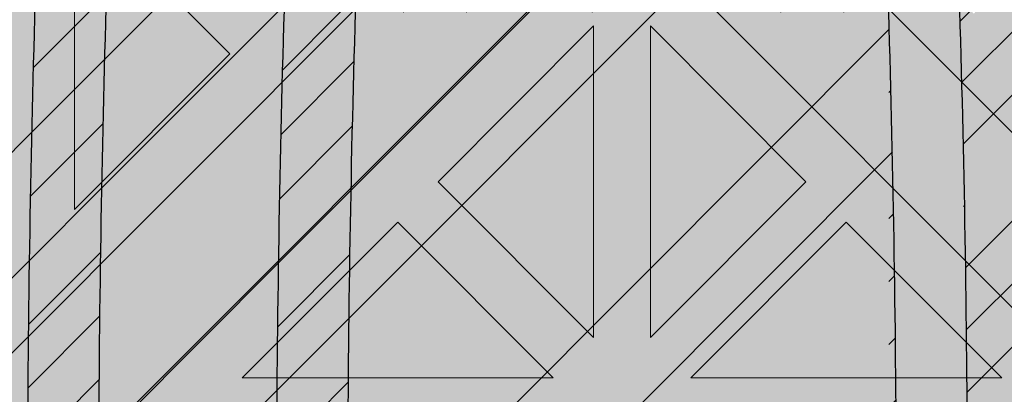
# Model space of a CAD drawing. Units: inches. Extents: x 844 to 2234, y 346 to 1084.
# Tile 60 of 93: x 1866.641 to 1871.054, y 703.938 to 705.614. Entities that reach past the tile are written whole.
import ezdxf

# ---------------------------------------------------------------- set-up
doc = ezdxf.new("R2010")
doc.units = ezdxf.units.IN
doc.header["$MEASUREMENT"] = 0
doc.layers.add('furniture', color=8, linetype='Continuous', lineweight=18)
doc.layers.add('RA-AP-01$0$INT', color=35, linetype='Continuous', lineweight=5)
doc.layers.add('RA-AP-01$0$FURN', color=3, linetype='Continuous')
doc.layers.add('RA-AP-01$0$WOOD', color=64, linetype='Continuous')

# ---------------------------------------------------------------- blocks, each defined once
blk = doc.blocks.new('A$C18D01794')
at = {"layer": 'RA-AP-01$0$INT'}
h = blk.add_hatch(color=256, dxfattribs=at)
h.paths.add_polyline_path([(4.585917135068448, -7.856712009587804), (4.614201406330596, -7.856712009587056), (4.668846067270487, -7.802067348644738), (4.723490728212344, -7.856712009584164), (4.771774999457151, -7.856712009582887), (4.826419660396886, -7.80206734864072), (4.862780050090322, -7.838427738332541), (4.844495778842715, -7.856712009580965), (4.862780050090411, -7.856712009580482), (4.905206456960182, -7.814285602707865), (4.947632863832445, -7.856712009578238), (4.965917135079675, -7.856712009577755), (4.947632863831759, -7.838427738330656), (4.983993253523576, -7.802067348637219), (5.038637914464627, -7.856712009575829), (5.08692218571208, -7.856712009574554), (5.141566846649976, -7.802067348634224), (5.196211507589851, -7.856712009571666), (5.224495778822615, -7.856712009570916), (4.905206456953975, -7.537422687702283)])
h.paths.add_polyline_path([(4.895206456956031, -7.575706958950402), (4.895206456958921, -7.684996280828174), (4.840561796018589, -7.630351619890275)], flags=16)
h.paths.add_polyline_path([(4.915206456955638, -7.575706958949956), (4.969851117895509, -7.630351619887399), (4.915206456957609, -7.684996280827732)], flags=16)
h.paths.add_polyline_path([(4.826419660395175, -7.644493755514321), (4.881064321335613, -7.699138416452331), (4.771774999456703, -7.69913841645522)], flags=16)
h.paths.add_polyline_path([(4.983993253519558, -7.644493755510815), (5.038637914460456, -7.699138416449285), (4.929348592581548, -7.69913841645126)], flags=16)
h.paths.add_polyline_path([(4.881064321336025, -7.719138416452334), (4.826419660397532, -7.773783077393256), (4.771774999457062, -7.719138416455217)], flags=16)
h.paths.add_polyline_path([(4.929348592582019, -7.71913841645126), (5.038637914460982, -7.719138416449284), (4.983993253522945, -7.773783077389749)], flags=16)
h.paths.add_polyline_path([(4.895206456960191, -7.733280552075633), (4.895206456962115, -7.806001331460164), (4.876922185715016, -7.824285602708492), (4.840561796021581, -7.787925213016675)], flags=16)
h.paths.add_polyline_path([(4.915206456958487, -7.733280552075187), (4.969851117899527, -7.787925213013798), (4.933490728206909, -7.824285602708034), (4.9152064569598, -7.806001331461736)], flags=16)
h.paths.add_polyline_path([(4.757632863832376, -7.733280552079264), (4.812277524772842, -7.787925213017304), (4.757632863834348, -7.842569873958233)], flags=16)
h.paths.add_polyline_path([(4.737632863832376, -7.73328055207979), (4.737632863834348, -7.842569873958701), (4.682988202893906, -7.787925213020692)], flags=16)
h.paths.add_polyline_path([(5.05278005008503, -7.733280552072701), (5.052780050087917, -7.842569873951664), (4.998135389146995, -7.787925213013169)], flags=16)
h.paths.add_polyline_path([(5.072780050085024, -7.733280552072333), (5.127424711025931, -7.787925213010806), (5.072780050087916, -7.842569873951244)], flags=16)
h.paths.add_polyline_path([(4.935917135072783, -7.506712009583784), (5.255206456948811, -7.826001331459767), (5.255206456948932, -7.797717060211899), (5.200561796010279, -7.743072399273238), (5.255206456949403, -7.688427738334128), (5.25520645694961, -7.640143467086677), (5.200561796009787, -7.585498806146837), (5.236922185702417, -7.549138416454212), (5.255206456949919, -7.56742268770172), (5.255206456949998, -7.549138416454178), (5.212780050078687, -7.506712009583814), (5.25520645695036, -7.464285602712145), (5.255206456950438, -7.446001331464763), (5.236922185702424, -7.464285602712779), (5.200561796009796, -7.427925213020149), (5.255206456950753, -7.373280552079203), (5.25520645695096, -7.324996280834394), (5.200561796010322, -7.270351619893748), (5.255206456951428, -7.215706958952649), (5.255206456951547, -7.187422687705071)])
h.paths.add_polyline_path([(5.042988202883395, -7.42792521302065), (5.097632863823085, -7.373280552080975), (5.097632863822622, -7.482569873959883)], flags=16)
h.paths.add_polyline_path([(5.028846067259663, -7.442067348644384), (5.083490728198774, -7.496712009583504), (4.974201406321001, -7.496712009583035)], flags=16)
h.paths.add_polyline_path([(5.117632863823087, -7.37328055208089), (5.172277524762331, -7.42792521302015), (5.11763286382262, -7.482569873959851)], flags=16)
h.paths.add_polyline_path([(5.08349072819877, -7.516712009582191), (5.028846067259652, -7.571356670521302), (4.974201406320998, -7.516712009582638)], flags=16)
h.paths.add_polyline_path([(5.131774999446817, -7.35913841645716), (5.186419660386065, -7.413783077396415), (5.241064321325782, -7.359138416456712)], flags=17)
h.paths.add_polyline_path([(5.131774999446228, -7.496712009583703), (5.186419660386065, -7.442067348643883), (5.222780050079488, -7.478427738337313), (5.204495778832781, -7.496712009584014)], flags=16)
h.paths.add_polyline_path([(5.097632863822613, -7.530854145205813), (5.097632863823061, -7.640143467084723), (5.042988202883383, -7.585498806145032)], flags=16)
h.paths.add_polyline_path([(5.131774999446899, -7.339138416457162), (5.241064321325809, -7.339138416456712), (5.186419660386591, -7.284493755517479)], flags=17)
h.paths.add_polyline_path([(5.131774999446226, -7.516712009581999), (5.204495778830767, -7.516712009581702), (5.22278005007868, -7.534996280829206), (5.186419660386049, -7.571356670521828)], flags=16)
h.paths.add_polyline_path([(5.11763286382262, -7.530854145205852), (5.17227752476232, -7.585498806145562), (5.117632863823064, -7.64014346708481)], flags=16)
h.paths.add_polyline_path([(5.186419660386069, -7.599640941770585), (5.241064321325754, -7.654285602710281), (5.131774999446791, -7.654285602709814)], flags=16)
h.paths.add_polyline_path([(5.131774999446872, -7.674285602709813), (5.24106432132578, -7.674285602710282), (5.186419660386554, -7.728930263649504)], flags=16)
h.paths.add_polyline_path([(5.255206456951811, -7.126001331467467), (5.255206456951895, -7.106712009588038), (4.555206456956052, -7.106712009588038), (4.555206456956136, -7.12600133146746), (4.905206456953973, -7.476001331465289)])
h.paths.add_polyline_path([(4.983993253513404, -7.368930263651977), (4.92934859257295, -7.314285602713969), (5.03863791445186, -7.314285602711063)], flags=16)
h.paths.add_polyline_path([(4.969851117889988, -7.383072399276016), (4.915206456952556, -7.437717060215906), (4.915206456949648, -7.328427738338133)], flags=16)
h.paths.add_polyline_path([(4.929348592572535, -7.294285602713971), (4.983993253511019, -7.239640941773039), (5.038637914451496, -7.294285602711065)], flags=16)
h.paths.add_polyline_path([(5.052780050074912, -7.280143467087016), (4.998135389134438, -7.225498806148989), (5.052780050072919, -7.170854145208052)], flags=16)
h.paths.add_polyline_path([(5.07278005007491, -7.280143467086489), (5.072780050072918, -7.170854145207579), (5.127424711013374, -7.225498806145578)], flags=16)
h.paths.add_polyline_path([(4.89520645695295, -7.437717060216355), (4.840561796013067, -7.383072399278919), (4.895206456950961, -7.328427738338582)], flags=16)
h.paths.add_polyline_path([(4.915206456948365, -7.280143467090674), (4.915206456946434, -7.207422687704125), (4.933490728192729, -7.18913841645701), (4.969851117886972, -7.225498806149623)], flags=16)
h.paths.add_polyline_path([(4.881064321327021, -7.314285602715054), (4.82641966038902, -7.368930263655506), (4.771774999448108, -7.314285602717047)], flags=16)
h.paths.add_polyline_path([(4.895206456950073, -7.280143467091125), (4.840561796009022, -7.225498806152518), (4.876922185700835, -7.18913841645908), (4.895206456948749, -7.207422687706589)], flags=16)
h.paths.add_polyline_path([(4.983993253510392, -7.211356670525576), (4.947632863816944, -7.174996280833758), (4.965917135064043, -7.156712009585847), (5.038637914448995, -7.156712009584522)], flags=16)
h.paths.add_polyline_path([(4.881064321326543, -7.294285602715056), (4.771774999447578, -7.294285602717046), (4.826419660385607, -7.239640941776569)], flags=16)
h.paths.add_polyline_path([(4.905206456946447, -7.19913841645844), (4.862780050074785, -7.156712009587725), (4.947632863816685, -7.156712009586302)], flags=16)
h.paths.add_polyline_path([(5.14156684663679, -7.211356670521528), (5.086922185696452, -7.156712009583639), (5.196211507574223, -7.156712009581651)], flags=16)
h.paths.add_polyline_path([(4.8264196603837, -7.211356670529104), (4.771774999442643, -7.156712009590501), (4.8444957788276, -7.156712009588568), (4.862780050075511, -7.17499628083566)], flags=16)
h.paths.add_polyline_path([(4.812277524760289, -7.225498806153156), (4.757632863822258, -7.28014346709363), (4.757632863819352, -7.170854145214669)], flags=16)
h.paths.add_polyline_path([(4.73763286382226, -7.280143467093997), (4.682988202881349, -7.22549880615554), (4.737632863819352, -7.170854145215086)], flags=16)
h.paths.add_polyline_path([(4.723490728195188, -7.156712009591787), (4.668846067257299, -7.211356670532127), (4.614201406317417, -7.156712009594693)], flags=16)
h.paths.add_polyline_path([(4.597632863829262, -7.506712009583814), (4.555206456957951, -7.54913841645418), (4.555206456958029, -7.56742268770172), (4.573490728205535, -7.549138416454212), (4.609851117898167, -7.585498806146839), (4.555206456958338, -7.640143467086675), (4.555206456958546, -7.688427738334125), (4.60985111789767, -7.743072399273238), (4.555206456959015, -7.797717060211899), (4.555206456959138, -7.826001331459767), (4.874495778835167, -7.506712009583786), (4.5552064569564, -7.187422687705062), (4.555206456956523, -7.215706958952644), (4.609851117897629, -7.270351619893746), (4.555206456956988, -7.324996280834396), (4.555206456957198, -7.373280552079195), (4.609851117898153, -7.427925213020147), (4.573490728205528, -7.464285602712779), (4.555206456957507, -7.446001331464756), (4.555206456957585, -7.464285602712143)])
h.paths.add_polyline_path([(4.712780050085332, -7.482569873959882), (4.712780050084863, -7.373280552080972), (4.767424711024555, -7.42792521302065)], flags=16)
h.paths.add_polyline_path([(4.726922185709173, -7.496712009583504), (4.781566846648288, -7.442067348644384), (4.836211507586949, -7.496712009583033)], flags=16)
h.paths.add_polyline_path([(4.692780050085327, -7.482569873959851), (4.638135389145619, -7.427925213020149), (4.692780050084865, -7.373280552080892)], flags=16)
h.paths.add_polyline_path([(4.726922185709182, -7.516712009582191), (4.836211507586949, -7.51671200958264), (4.7815668466483, -7.571356670521304)], flags=16)
h.paths.add_polyline_path([(4.678637914461726, -7.496712009583706), (4.605917135075169, -7.496712009584014), (4.587632863828464, -7.478427738337311), (4.623993253521887, -7.442067348643881)], flags=16)
h.paths.add_polyline_path([(4.712780050085336, -7.530854145205816), (4.767424711024568, -7.585498806145034), (4.71278005008489, -7.640143467084724)], flags=16)
h.paths.add_polyline_path([(4.678637914461726, -7.516712009582001), (4.623993253521899, -7.571356670521829), (4.587632863829271, -7.534996280829206), (4.605917135077185, -7.5167120095817)], flags=16)
h.paths.add_polyline_path([(4.692780050085336, -7.530854145205848), (4.692780050084889, -7.64014346708481), (4.638135389145632, -7.585498806145562)], flags=16)
h.paths.add_polyline_path([(4.623993253521885, -7.413783077396415), (4.678637914461131, -7.359138416457161), (4.56934859258217, -7.359138416456712)], flags=17)
h.paths.add_polyline_path([(4.623993253521901, -7.599640941770568), (4.678637914461158, -7.654285602709814), (4.569348592582195, -7.654285602710281)], flags=16)
h.paths.add_polyline_path([(4.678637914461051, -7.339138416457162), (4.623993253521361, -7.284493755517479), (4.569348592582143, -7.339138416456712)], flags=17)
h.paths.add_polyline_path([(4.678637914461076, -7.674285602709813), (4.623993253521399, -7.728930263649504), (4.569348592582167, -7.674285602710281)], flags=16)
h = blk.add_hatch(color=256, dxfattribs=at)
h.paths.add_polyline_path([(4.905206456954232, -7.537422687702028), (4.874495778835232, -7.506712009583718), (4.555206456959138, -7.826001331459766), (4.555206456959269, -7.856712009588616), (4.585917135068449, -7.856712009587804)])
h.paths.add_polyline_path([(4.935917135072152, -7.506712009583152), (4.905206456953497, -7.537422687701806), (5.224495778822614, -7.856712009570917), (5.255206456948681, -7.856712009570104), (5.255206456948813, -7.826001331459768)])
h.paths.add_polyline_path([(5.255206456951549, -7.18742268770507), (5.255206456951813, -7.126001331467461), (4.905206456953563, -7.476001331465701), (4.935917135072559, -7.506712009584006)])
h.paths.add_polyline_path([(4.874495778835167, -7.506712009583785), (4.905206456953818, -7.476001331465132), (4.555206456956135, -7.126001331467458), (4.555206456956399, -7.187422687705064)])
h = blk.add_hatch(color=256, dxfattribs=at)
h.paths.add_polyline_path([(4.89520645695096, -7.328427738338579), (4.840561796013068, -7.383072399278921), (4.89520645695295, -7.437717060216353)])
h.paths.add_polyline_path([(4.915206456952557, -7.437717060215907), (4.969851117889986, -7.383072399276024), (4.915206456949648, -7.328427738338133)])
h.paths.add_polyline_path([(4.929348592572952, -7.31428560271397), (4.983993253513403, -7.368930263651974), (5.038637914451863, -7.314285602711064)])
h.paths.add_polyline_path([(5.038637914451498, -7.294285602711065), (4.983993253511018, -7.239640941773039), (4.929348592572535, -7.294285602713969)])
h.paths.add_polyline_path([(4.969851117886971, -7.225498806149624), (4.93349072819273, -7.189138416457011), (4.915206456946433, -7.207422687704124), (4.915206456948367, -7.280143467090678)])
h.paths.add_polyline_path([(4.965917135064045, -7.156712009585847), (4.947632863816945, -7.17499628083376), (4.983993253510389, -7.211356670525573), (5.038637914448995, -7.156712009584522)])
h.paths.add_polyline_path([(4.998135389134439, -7.22549880614899), (5.05278005007491, -7.280143467087016), (5.052780050072921, -7.170854145208054)])
h.paths.add_polyline_path([(5.072780050074911, -7.28014346708649), (5.127424711013374, -7.225498806145579), (5.072780050072921, -7.170854145207581)])
h.paths.add_polyline_path([(5.196211507574225, -7.156712009581651), (5.08692218569645, -7.156712009583639), (5.141566846636789, -7.211356670521529)])
h.paths.add_polyline_path([(4.862780050074782, -7.156712009587723), (4.90520645694645, -7.199138416458444), (4.94763286381669, -7.156712009586302)])
h.paths.add_polyline_path([(4.895206456950073, -7.280143467091126), (4.895206456948746, -7.207422687706587), (4.876922185700836, -7.189138416459078), (4.840561796009025, -7.225498806152521)])
h.paths.add_polyline_path([(4.826419660385605, -7.239640941776569), (4.771774999447577, -7.294285602717049), (4.881064321326541, -7.294285602715055)])
h.paths.add_polyline_path([(4.771774999448108, -7.314285602717046), (4.82641966038902, -7.368930263655505), (4.88106432132702, -7.314285602715054)])
h.paths.add_polyline_path([(4.757632863822258, -7.280143467093631), (4.812277524760285, -7.225498806153153), (4.757632863819352, -7.170854145214668)])
h.paths.add_polyline_path([(4.862780050075512, -7.17499628083566), (4.844495778827599, -7.156712009588567), (4.771774999442647, -7.156712009590504), (4.8264196603837, -7.211356670529104)])
h.paths.add_polyline_path([(4.682988202881349, -7.225498806155537), (4.737632863822258, -7.280143467093997), (4.737632863819352, -7.170854145215087)])
h.paths.add_polyline_path([(4.723490728195189, -7.156712009591783), (4.614201406317418, -7.156712009594692), (4.668846067257298, -7.211356670532127)])
h = blk.add_hatch(color=256, dxfattribs=at)
h.paths.add_polyline_path([(4.781566846647504, -7.442067348645805), (4.836211507586161, -7.496712009584463), (4.726922185708388, -7.496712009584918)])
h.paths.add_polyline_path([(4.836211507586161, -7.516712009584068), (4.781566846647504, -7.571356670522723), (4.726922185708388, -7.516712009583606)])
h.paths.add_polyline_path([(4.76742471102377, -7.585498806146453), (4.712780050084083, -7.640143467086137), (4.712780050084542, -7.530854145207227)])
h.paths.add_polyline_path([(4.692780050084544, -7.530854145207257), (4.692780050084084, -7.64014346708622), (4.638135389144834, -7.585498806146965)])
h.paths.add_polyline_path([(4.678637914460932, -7.516712009583407), (4.623993253521102, -7.571356670523233), (4.587632863827676, -7.53499628082981), (4.605917135074382, -7.516712009583104)])
h.paths.add_polyline_path([(4.573490728204743, -7.54913841645434), (4.60985111789737, -7.585498806146969), (4.555206456957541, -7.640143467086797), (4.555206456957237, -7.567422687701846)])
h.paths.add_polyline_path([(4.623993253521098, -7.599640941770699), (4.67863791446035, -7.654285602709951), (4.56934859258139, -7.654285602710407)])
h.paths.add_polyline_path([(4.678637914460275, -7.67428560270995), (4.623993253520583, -7.728930263649637), (4.56934859258136, -7.674285602710405)])
h.paths.add_polyline_path([(4.609851117896854, -7.743072399273369), (4.555206456958196, -7.797717060212026), (4.555206456957738, -7.688427738334254)])
h.paths.add_polyline_path([(4.597632863828475, -7.506712009583301), (4.555206456957283, -7.549138416454495), (4.555206456956805, -7.464285602712587)])
h.paths.add_polyline_path([(4.678637914460932, -7.496712009585113), (4.605917135076396, -7.496712009585417), (4.587632863828479, -7.478427738337913), (4.623993253521104, -7.442067348645284)])
h.paths.add_polyline_path([(4.692780050084091, -7.373280552082301), (4.692780050084548, -7.482569873961267), (4.638135389144834, -7.427925213021552)])
h.paths.add_polyline_path([(4.767424711023772, -7.427925213022072), (4.712780050084545, -7.48256987396129), (4.712780050084089, -7.373280552082384)])
h.paths.add_polyline_path([(4.67863791446036, -7.359138416457298), (4.623993253521105, -7.41378307739655), (4.569348592581399, -7.35913841645684)])
h.paths.add_polyline_path([(4.609851117897371, -7.427925213020278), (4.573490728204743, -7.464285602712907), (4.555206456957237, -7.446001331465401), (4.555206456957548, -7.373280552080448)])
h.paths.add_polyline_path([(4.623993253520596, -7.284493755517612), (4.67863791446028, -7.339138416457299), (4.569348592581367, -7.339138416456838)])
h.paths.add_polyline_path([(4.609851117896867, -7.270351619893878), (4.555206456957749, -7.324996280832994), (4.55520645695821, -7.21570695895522)])
for p, q in [((4.905206456953975, -7.476001331465289), (4.555206456956136, -7.12600133146746)), ((4.905206456953975, -7.476001331465289), (5.255206456951811, -7.126001331467465)), ((4.874495778835167, -7.506712009583786), (4.555206456956399, -7.187422687705064)), ((4.935917135072783, -7.506712009583784), (5.255206456951548, -7.187422687705069)), ((4.771774999448109, -7.314285602717045), (4.881064321327019, -7.314285602715054)), ((4.826419660389018, -7.368930263655503), (4.771774999448109, -7.314285602717045)), ((4.881064321327019, -7.314285602715054), (4.82641966038902, -7.368930263655505)), ((4.929348592572952, -7.314285602713971), (4.983993253513403, -7.368930263651975)), ((5.038637914451862, -7.314285602711064), (4.929348592572952, -7.314285602713971)), ((4.983993253513404, -7.368930263651973), (5.038637914451862, -7.314285602711064)), ((4.895206456950956, -7.328427738338584), (4.840561796013068, -7.383072399278921)), ((4.895206456950959, -7.328427738338582), (4.89520645695295, -7.437717060216353)), ((4.915206456949651, -7.328427738338136), (4.969851117889986, -7.383072399276024)), ((4.915206456949648, -7.328427738338135), (4.915206456952556, -7.437717060215906)), ((4.767424711024554, -7.42792521302065), (4.712780050084865, -7.373280552080972)), ((4.712780050084865, -7.373280552080972), (4.71278005008533, -7.482569873959882)), ((4.89520645695295, -7.437717060216353), (4.840561796013068, -7.383072399278921)), ((4.915206456952556, -7.437717060215906), (4.969851117889986, -7.383072399276024)), ((4.71278005008533, -7.482569873959882), (4.767424711024555, -7.427925213020651))]:
    blk.add_line(p, q, dxfattribs=at)
blk = doc.blocks.new('A$C32926AE1')
at = {"layer": 'RA-AP-01$0$FURN'}
h = blk.add_hatch(dxfattribs=at)
h.set_pattern_fill('ANSI31', color=256, scale=0.1, style=0)
h.set_pattern_definition([(45, (0, 0), (-0.0088388347648318, 0.0088388347648318), [])])
edge = h.paths.add_edge_path(flags=16)
edge.add_arc((4.904771284329206, 4.246793130718756), 0.2603971832811541, 75.22398030683196, 104.7760196931204)
edge.add_arc((4.904771284329206, 4.246793130718756), 0.2603971832811541, 75.223980306832, 104.77601969312039, ccw=False)
edge = h.paths.add_edge_path(flags=16)
edge.add_arc((4.904771284329206, 4.067062675376612), 0.2603971832811541, 255.2239803068796, 284.776019693168)
edge.add_arc((4.904771284329206, 4.067062675376612), 0.2603971832811541, 255.22398030687958, 284.77601969316805, ccw=False)
edge = h.paths.add_edge_path(flags=0)
edge.add_arc((4.904771284329206, 4.067062675376612), 0.2603971832811541, 255.2239803068796, 284.776019693168)
edge.add_arc((4.904771284329206, 4.067062675376612), 0.2603971832811541, 255.22398030687958, 284.77601969316805, ccw=False)
edge = h.paths.add_edge_path(flags=0)
edge.add_arc((4.904771284329206, 4.067062675376612), 0.2603971832811541, 255.2239803068796, 284.776019693168)
edge.add_arc((4.904771284329206, 4.067062675376612), 0.2603971832811541, 255.22398030687958, 284.77601969316805, ccw=False)
edge = h.paths.add_edge_path()
edge.add_arc((4.604388392048174, 4.588829985554312), 0.1599999999999918, 342.3781640246255, 354.4317409793762)
edge.add_arc((5.090145208887507, 4.43216705527679), 0.3503971832811637, 162.0091218307731, 180.3186872093483)
edge.add_arc((5.205154176610243, 4.588829985554953), 0.1599999999999917, 185.5682590208461, 197.6218359767349)
edge.add_arc((4.904771284329229, 4.246793130718735), 0.3503971832811761, 72.00912183053516, 107.9908781690354)
edge.add_arc((9.535952835716557, 4.28682295566602), 4.798342501046485, 178.2875002453811, 181.5576802719453)
edge.add_arc((4.719397359771122, 4.43216705527679), 0.3503971832811637, 359.6813127906516, 377.9908781692269)
edge.add_arc((9.535967292294904, 4.286822350292874), 4.778371420254705, 178.2965938931842, 181.5667745797229)
edge.add_arc((4.719397359771122, 4.43216705527679), 0.3303971832811637, 359.6813127906516, 377.9908781692269)
edge.add_arc((0.2735752763637294, 4.286822350292874), 4.7783714202547, 358.4332254202771, 361.7034061068158)
edge.add_arc((5.061434214606998, 4.732549947558029), 0.1600000000000254, 252.3781640250584, 264.4317409792362)
edge.add_arc((4.748108354051257, 4.732549947558012), 0.1600000000000541, 275.5682590208426, 287.6218359759532)
edge.add_arc((4.604388392048115, 4.588829985554317), 0.1800000000000505, 342.3567572500182, 349.3735009646207)
edge.add_arc((5.205154176610254, 4.588829985554976), 0.1800000000000069, 190.6264990356027, 197.6432427513933)
edge.add_arc((5.061434214607106, 4.732549947558013), 0.1800000000000424, 252.3567572496606, 259.3735009644582)
edge.add_arc((4.904771284329208, 4.246793130718737), 0.3303971832811676, 71.99844483668534, 108.0015551637021)
edge.add_arc((4.748108354051414, 4.732549947558045), 0.1800000000000547, 280.6264990355479, 287.6432427495938)
edge.add_arc((5.090145208887514, 4.432167055276789), 0.2803971832811691, 162.8706300666893, 180.816523289902)
edge.add_arc((4.719397359771136, 4.432167055276689), 0.2803971832811534, 359.183476710103, 377.1293699333214)
edge.add_arc((4.904771284329222, 4.246793130718737), 0.2803971832811769, 72.87063006672916, 107.1293699332334)
edge.add_arc((5.090145208887522, 4.432167055276788), 0.2603971832811776, 165.2239803068007, 180.9953123810312)
edge.add_arc((4.719397359771141, 4.432167055276699), 0.2603971832811458, 359.0046876189768, 374.7760196932087)
edge.add_arc((5.090145208887507, 4.43216705527679), 0.3303971832811637, 162.0091218307731, 180.3186872093483)
edge.add_arc((9.53595427642584, 4.285015535491528), 4.728345371032053, 178.265043920078, 181.5679956281801)
edge.add_arc((0.2735882922327999, 4.285015535491582), 4.728345371032045, 358.4320043718193, 361.7349560799204)
edge.add_arc((9.535953591267507, 4.284458026472751), 4.708343996644348, 178.2573054306777, 181.5704995759608)
edge.add_arc((0.273588977391114, 4.284458026472785), 4.708343996644358, 358.4295004240388, 361.7426945693213)
edge.add_arc((0.2735889773911131, 4.029397779622582), 4.708343996644359, 358.2573054306787, 361.5704995759613)
edge.add_arc((9.535953591267518, 4.029397779622618), 4.708343996644359, 178.4295004240391, 181.7426945693223)
edge.add_arc((0.2735882922327901, 4.028840270603786), 4.728345371032054, 358.2650439200796, 361.5679956281808)
edge.add_arc((9.53595427642584, 4.028840270603841), 4.728345371032054, 178.4320043718199, 181.7349560799219)
edge.add_arc((0.2735752763637302, 4.027033455802493), 4.778371420254699, 358.2965938931842, 361.5667745797229)
edge.add_arc((4.719397359771122, 3.881688750818578), 0.3303971832811637, 342.0091218307731, 360.3186872093484)
edge.add_arc((5.090145208887507, 3.881688750818578), 0.3303971832811637, 179.6813127906516, 197.9908781692269)
edge.add_arc((9.535967292294904, 4.027033455802493), 4.778371420254705, 178.433225420277, 181.7034061068158)
edge.add_arc((4.719397359771122, 3.881688750818578), 0.3503971832811637, 342.0091218307731, 360.3186872093484)
edge.add_arc((9.53595283571655, 4.027032850429349), 4.79834250104648, 178.4423197280546, 181.7124997546188)
edge.add_arc((4.719397359771141, 3.881688750818669), 0.2603971832811458, 345.2239803067913, 360.9953123810232)
edge.add_arc((5.090145208887522, 3.88168875081858), 0.2603971832811776, 179.0046876189687, 194.7760196931993)
edge.add_arc((4.904771284329222, 4.067062675376631), 0.2803971832811769, 252.8706300667665, 287.1293699332708)
edge.add_arc((4.719397359771136, 3.881688750818678), 0.2803971832811534, 342.8706300666787, 360.8165232898969)
edge.add_arc((5.090145208887514, 3.881688750818579), 0.2803971832811691, 179.183476710098, 197.1293699333106)
edge.add_arc((4.748108354051414, 3.581305858537323), 0.1800000000000547, 72.3567572504062, 79.37350096445199)
edge.add_arc((4.904771284329208, 4.067062675376631), 0.3303971832811676, 251.9984448362979, 288.0015551633146)
edge.add_arc((5.061434214607106, 3.581305858537355), 0.1800000000000424, 100.6264990355418, 107.6432427503394)
edge.add_arc((5.205154176610254, 3.725025820540392), 0.1800000000000069, 162.3567572486066, 169.3735009643972)
edge.add_arc((4.604388392048115, 3.725025820541051), 0.1800000000000505, 10.62649903537925, 17.64324274998182)
edge.add_arc((4.748108354051257, 3.581305858537356), 0.1600000000000541, 72.37816402404681, 84.43174097915735)
edge.add_arc((4.904771284329229, 4.067062675376632), 0.3503971832811761, 252.0091218309645, 287.9908781694648)
edge.add_arc((5.061434214606998, 3.581305858537339), 0.1600000000000254, 95.56825902076373, 107.6218359749416)
edge.add_arc((5.205154176610243, 3.725025820540414), 0.1599999999999917, 162.3781640232651, 174.4317409791539)
edge.add_arc((5.090145208887507, 3.881688750818578), 0.3503971832811637, 179.6813127906516, 197.9908781692269)
edge.add_arc((4.604388392048174, 3.725025820541056), 0.1599999999999918, 5.568259020623824, 17.62183597537444)
edge.add_arc((0.2735897329420762, 4.28682295566602), 4.798342501046482, 358.4423197280547, 361.7124997546188)
edge.add_arc((0.2735897329420691, 4.027032850429348), 4.798342501046489, 358.2875002453812, 361.5576802719453)
at = {"layer": 'RA-AP-01$0$WOOD'}
h = blk.add_hatch(color=256, dxfattribs=at)
h.dxf.hatch_style = 1
h.paths.add_polyline_path([(5.157430609644524, 4.573483066760929, -0.1009492694046607), (5.155401577623758, 4.593365984175333, -0.1842662638101597), (5.172249623284174, 4.638795604568598, 0.2056608120311276), (5.179560981299304, 4.661316324430096, 0.3614336704623542), (5.134352340494423, 4.706524965234944, 0.2056608120311297), (5.111831620632933, 4.699213607219793, -0.1842662638101113), (5.066402000239693, 4.682365561559342, -0.1055311479399994), (5.045656153913092, 4.68467289944697, 0.1567636581983829), (4.763886414745334, 4.684672899446966, -0.1055311479399895), (4.743140568418733, 4.68236556155934, -0.1842662638100833), (4.6977109480255, 4.69921360721979, 0.2056608120302612), (4.675190228164109, 4.706524965234949, 0.3614336704708441), (4.629981587358889, 4.66131632442871, 0.2056608120245944), (4.637292945374126, 4.638795604567974, -0.1842662638101024), (4.654140991034615, 4.59336598417475, -0.1009492694055169), (4.652111959013835, 4.573483066760181, 0.021410119221476), (4.629748025606143, 4.156712009541676, 0.0214101192214795), (4.652111959013809, 3.739940952323101, -0.1009492694059586), (4.654140991034615, 3.720058034908448, -0.1842662638100975), (4.637292945374126, 3.674628414515226, 0.2056608120245705), (4.629981587358889, 3.652107694654492, 0.3614336704708879), (4.675190228164113, 3.606899053848249, 0.2056608120302384), (4.697710948025501, 3.614210411863408, -0.1842662638100995), (4.743140568418738, 3.63105845752386, -0.1055311479402541), (4.763886414745388, 3.628751119636215, 0.1567636581983776), (5.045656153913137, 3.628751119636244, -0.1055311479397538), (5.066402000239692, 3.631058457523857, -0.1842662638101067), (5.111831620632931, 3.614210411863407, 0.2056608120310924), (5.134352340494417, 3.606899053848256, 0.3614336704624001), (5.179560981299307, 3.652107694653103, 0.2056608120311314), (5.172249623284175, 3.6746284145146, -0.1842662638101402), (5.155401577623758, 3.72005803490786, -0.1009492694051366), (5.15743060964455, 3.739940952322354, 0.0214101192215073), (5.179794543052287, 4.156712009541468, 0.0214101192215252)])
h.paths.add_polyline_path([(4.639748609479751, 4.156712009541513, 0.0213537860821624), (4.661970494867118, 3.741887061152232, -0.094075836301374), (4.664143710413708, 3.7196126951003, -0.1824818158568985), (4.644813765429836, 3.668037719127816, 0.2056608120245319), (4.639939526753007, 3.653023905887301, 0.3614336704710246), (4.676106439397173, 3.616856993242342, 0.2056608120302234), (4.691120252638095, 3.621731231919122, -0.1824818158602558), (4.742695228611606, 3.641061176902986, -0.1029891339458722), (4.766991894714349, 3.638256818950944, 0.156709409989566), (5.042550673941472, 3.638256818950105, -0.102989133958497), (5.066847340047078, 3.641061176902949, -0.1824818158594995), (5.118422316020358, 3.621731231919103, 0.2056608120311416), (5.133436129261316, 3.616856993242346, 0.3614336704621468), (5.169603041905217, 3.653023905886178, 0.2056608120310986), (5.164728803228477, 3.668037719127177, -0.1824818158565612), (5.145398858244737, 3.719612695099578, -0.0940758363009313), (5.147572073791232, 3.741887061151398, 0.0213537860822023), (5.169793959178681, 4.156712009541451, 0.0213537860822226), (5.147572073791203, 4.571536957931898, -0.0940758363005034), (5.145398858244737, 4.59381132398362, -0.1824818158565587), (5.164728803228476, 4.645386299956021, 0.2056608120311045), (5.169603041905216, 4.66040011319702, 0.3614336704621845), (5.133436129261313, 4.696567025840856, 0.2056608120310773), (5.118422316020359, 4.691692787164098, -0.182481815859508), (5.066847340047078, 4.67236284218025, -0.1029891339584606), (5.04255067394148, 4.675167200133092, 0.156709409989566), (4.766991894714357, 4.675167200132257, -0.1029891339458842), (4.742695228611611, 4.672362842180213, -0.1824818158602725), (4.691120252638095, 4.691692787164077, 0.2056608120302152), (4.676106439397174, 4.696567025840858, 0.3614336704710363), (4.639939526753005, 4.660400113195899, 0.2056608120245495), (4.644813765429837, 4.645386299955384, -0.1824818158568934), (4.664143710413708, 4.593811323982902, -0.0940758363009187), (4.661970494867149, 4.571536957931074, 0.021353786082177)], flags=16)
h.paths.add_polyline_path([(5.129794543052235, 4.432167055276933, -0.0141661062790638), (5.130152669293814, 4.156927903047693, -0.0141661062790647), (5.129794543052234, 3.881688750818433, -0.0785247771143638), (5.10979738006795, 3.755143611847103, 0.0945969212073497), (5.105408519571111, 3.717898134952927, 0.1043170707844957), (5.116074640131521, 3.670385395016088, 0.1043170707864965), (5.068561900193738, 3.681051515576561, 0.09459692119553), (5.031316423304057, 3.676662655080835, -0.1580239521427272), (4.778226145355827, 3.676662655080367, 0.0945969211986668), (4.740980668464973, 3.681051515576592, 0.1043170707882822), (4.693467928526415, 3.670385395015844, 0.1043170707867916), (4.704134049087309, 3.717898134953662, 0.0945969211972894), (4.69974518859162, 3.755143611844042, -0.0785247771163196), (4.679748025606343, 3.881688750818406, -0.0141661062790663), (4.679389899364763, 4.156927903047693, -0.0141661062790672), (4.679748025606343, 4.432167055276998, -0.0785247771163064), (4.699745188591625, 4.55871219425134, 0.094596921197333), (4.704134049087308, 4.595957671141738, 0.1043170707867205), (4.693467928526416, 4.643470411079523, 0.1043170707882628), (4.740980668464965, 4.632804290518776, 0.0945969211988114), (4.778226145355874, 4.637193151015016, -0.158023952142669), (5.031316423304015, 4.637193151014546, 0.0945969211956361), (5.068561900193736, 4.632804290518806, 0.1043170707864979), (5.11607464013152, 4.643470411079278, 0.1043170707844617), (5.105408519571112, 4.595957671142455, 0.0945969212074597), (5.109797380067959, 4.558712194248236, -0.0785247771143467)], flags=0)
h.paths.add_polyline_path([(5.119794532311105, 4.432259799204851, -0.0142000800617244), (5.120156169157484, 4.156927903047701, -0.0142000800617277), (5.119794532311105, 3.881596006890482, -0.0784894509520253), (5.100273383573699, 3.758192358677797, 0.0940138827242913), (5.095413455884425, 3.717477693979438, 0.0606271852308753), (5.099615656341024, 3.686844378806616, 0.0606271852322524), (5.068982341167493, 3.691046579263239, 0.0940138827010453), (5.028267676478798, 3.686186651576848, -0.1580706864508061), (4.781274892180912, 3.686186651576435, 0.0940138827026903), (4.740560227491556, 3.691046579263279, 0.0606271852339895), (4.709926912317155, 3.686844378806508, 0.0606271852329405), (4.714129112773991, 3.717477693980356, 0.094013882701304), (4.709269185087677, 3.758192358669163, -0.0784894509577193), (4.689748036347473, 3.881596006890469, -0.014200080061729), (4.689386399501094, 4.156927903047709, -0.0142000800617217), (4.689748036347473, 4.432259799204808, -0.078489450957724), (4.709269185087651, 4.555663447426125, 0.0940138827014585), (4.714129112773992, 4.596378112114996, 0.0606271852329731), (4.709926912317154, 4.62701142728886, 0.0606271852340196), (4.74056022749157, 4.622809226832087, 0.0940138827024997), (4.781274892180847, 4.627669154518912, -0.1580706864508359), (5.028267676478777, 4.627669154518526, 0.0940138827010946), (5.068982341167492, 4.622809226832129, 0.060627185232254), (5.099615656341024, 4.627011427288751, 0.0606271852308727), (5.095413455884425, 4.59637811211593, 0.0940138827241088), (5.100273383573675, 4.555663447417647, -0.0784894509520978)], flags=0)
h.paths.add_polyline_path([(5.06978912287499, 4.430218106756144, -0.014241683694547), (5.070173729147532, 4.156927903047672, -0.0142416836945458), (5.06978912287499, 3.883637699339223, -0.0800609523125196), (5.052662118612511, 3.773463122773442, 0.0526421978001116), (5.04590916754064, 3.740550867606997, 0.0526421977992423), (5.012996912374707, 3.73379791653534, -0.1583028414718258), (4.796545656286308, 3.73379791653451, 0.0526421978034211), (4.763633401117837, 3.740550867607021, 0.0526421978018622), (4.756880450045755, 3.773463122774558, -0.0800609523117106), (4.739753445783639, 3.883637699339268, -0.0142416836945435), (4.739368839511098, 4.156927903047671, -0.0142416836945477), (4.739753445783639, 4.430218106756155, -0.0800609523116345), (4.75688045004574, 4.540392683320762, 0.052642197801941), (4.763633401117837, 4.573304938488346, 0.0526421978035071), (4.796545656286361, 4.580057889560873, -0.1583028414717561), (5.012996912374669, 4.580057889560039, 0.0526421977993048), (5.04590916754064, 4.57330493848837, 0.0526421978002057), (5.052662118612529, 4.540392683321868, -0.080060952312477)], flags=0)
h.paths.add_polyline_path([(5.049789715110557, 4.43038092723357, -0.0143097550741839), (5.05018085590259, 4.156927903047715, -0.0143097550741854), (5.049789715110558, 3.883474878861827, -0.0800685599149176), (5.03362098255317, 3.779581877367999, 0.0306258898956367), (5.028241146483733, 3.758218888663947, 0.0306258898977031), (5.006878157778253, 3.75283905259408, -0.1583983521624096), (4.802664410878162, 3.752839052594731, 0.0306258898946014), (4.781301422174808, 3.758218888663924, 0.0306258898967912), (4.775921586105202, 3.779581877368794, -0.080068559914251), (4.759752853548071, 3.883474878861786, -0.0143097550741854), (4.759361712756037, 4.156927903047671, -0.0143097550741854), (4.759752853548071, 4.430380927233557, -0.0800685599142479), (4.775921586105193, 4.534273928726546, 0.0306258898968306), (4.781301422174808, 4.555636917431444, 0.0306258898945754), (4.802664410878143, 4.561016753500631, -0.1583983521624168), (5.006878157778244, 4.561016753501291, 0.0306258898977177), (5.028241146483733, 4.555636917431421, 0.0306258898958182), (5.03362098255321, 4.534273928727244, -0.080068559914796)], flags=0)
h.paths.add_polyline_path([(4.999766070382627, 4.428171244713864, -0.0143443147609634), (5.000198441819402, 4.156927903047689, -0.0143443147609612), (4.999766070382627, 3.885684561381556, -0.0784641635803329), (4.987356730658798, 3.799103304488872, -0.1506053783831347), (4.822185837999821, 3.79910330448882, -0.0784641635803318), (4.809776498276007, 3.885684561381509, -0.014344314760963), (4.809344126839227, 4.156927903047677, -0.0143443147609645), (4.809776498276007, 4.428171244713873, -0.0784641635803192), (4.822185837999822, 4.514752501606549, -0.1506053783831338), (4.987356730658798, 4.514752501606494, -0.078464163580285)], flags=0)
h.paths.add_polyline_path([(4.979755254238824, 4.42764379880488, -0.0143772539198268), (4.980205517789977, 4.156927903047693, -0.0143772539198275), (4.979755254238824, 3.886212007290489, -0.0689242507424422), (4.971183264704897, 3.815276770442801, -0.1296645318904179), (4.838359303953726, 3.815276770442746, -0.0689242507424186), (4.829787314419809, 3.886212007290419, -0.0143772539198292), (4.829337050868653, 4.156927903047653, -0.0143772539198325), (4.829787314419809, 4.427643798804946, -0.0689242507424211), (4.838359303953725, 4.498579035652621, -0.1296645318904187), (4.971183264704897, 4.498579035652565, -0.0689242507424401)], flags=0)
h = blk.add_hatch(color=256, dxfattribs=at)
h.dxf.hatch_style = 1
h.paths.add_polyline_path([(5.145398858244737, 4.59381132398362, -0.1824818158565616), (5.164728803228476, 4.645386299956021, 0.2056608120311045), (5.169603041905216, 4.66040011319702, 0.3614336704621845), (5.133436129261313, 4.696567025840856, 0.2056608120310773), (5.118422316020359, 4.691692787164098, -0.182481815859508), (5.066847340047078, 4.67236284218025, -0.1029891339584606), (5.04255067394148, 4.675167200133092, 0.156709409989566), (4.766991894714357, 4.675167200132257, -0.1029891339458842), (4.742695228611611, 4.672362842180213, -0.1824818158602725), (4.691120252638095, 4.691692787164077, 0.2056608120302152), (4.676106439397174, 4.696567025840858, 0.3614336704710363), (4.639939526753005, 4.660400113195899, 0.2056608120245495), (4.644813765429837, 4.645386299955384, -0.1824818158568934), (4.664143710413708, 4.593811323982902, -0.0940758363009187), (4.661970494867149, 4.571536957931074, 0.0213537860821772), (4.639748609479751, 4.156712009541507, 0.0213537860821625), (4.661970494867119, 3.741887061152226, -0.0940758363013071), (4.664143710413708, 3.719612695100309, -0.1824818158569294), (4.644813765429836, 3.668037719127816, 0.2056608120245319), (4.639939526753007, 3.653023905887301, 0.3614336704710246), (4.676106439397173, 3.616856993242342, 0.2056608120302234), (4.691120252638095, 3.621731231919122, -0.1824818158602558), (4.742695228611606, 3.641061176902986, -0.1029891339458722), (4.766991894714349, 3.638256818950944, 0.156709409989566), (5.042550673941472, 3.638256818950105, -0.102989133958497), (5.066847340047078, 3.641061176902949, -0.1824818158594995), (5.118422316020358, 3.621731231919103, 0.2056608120311416), (5.133436129261316, 3.616856993242346, 0.3614336704621468), (5.169603041905217, 3.653023905886178, 0.2056608120310986), (5.164728803228477, 3.668037719127177, -0.1824818158565612), (5.145398858244737, 3.719612695099578, -0.0940758363009313), (5.147572073791232, 3.741887061151398, 0.0213537860822023), (5.169793959178681, 4.156712009541451, 0.0213537860822226), (5.147572073791203, 4.571536957931898, -0.0940758363004996)])
h.paths.add_polyline_path([(5.109797380067958, 4.55871219424824, -0.0785247771143472), (5.129794543052234, 4.432167055276936, -0.0141661062790644), (5.130152669293814, 4.156927903047685, -0.014166106279066), (5.129794543052234, 3.881688750818401, -0.0785247771143517), (5.109797380067946, 3.755143611847092, 0.0945969212073132), (5.105408519571111, 3.717898134952929, 0.1043170707844995), (5.116074640131521, 3.670385395016088, 0.1043170707864965), (5.068561900193738, 3.681051515576561, 0.09459692119553), (5.031316423304057, 3.676662655080835, -0.1580239521427272), (4.778226145355827, 3.676662655080367, 0.0945969211986668), (4.740980668464973, 3.681051515576592, 0.1043170707882822), (4.693467928526415, 3.670385395015844, 0.1043170707867916), (4.704134049087309, 3.717898134953662, 0.0945969211972894), (4.69974518859162, 3.755143611844042, -0.0785247771163196), (4.679748025606343, 3.881688750818406, -0.0141661062790663), (4.679389899364763, 4.156927903047693, -0.0141661062790672), (4.679748025606343, 4.432167055276998, -0.0785247771163064), (4.699745188591625, 4.55871219425134, 0.094596921197333), (4.704134049087308, 4.595957671141738, 0.1043170707867205), (4.693467928526416, 4.643470411079523, 0.1043170707882628), (4.740980668464965, 4.632804290518776, 0.0945969211988114), (4.778226145355874, 4.637193151015016, -0.158023952142669), (5.031316423304015, 4.637193151014546, 0.0945969211956361), (5.068561900193736, 4.632804290518806, 0.1043170707864979), (5.11607464013152, 4.643470411079278, 0.1043170707844617), (5.105408519571112, 4.595957671142455, 0.0945969212074504)], flags=16)
h.paths.add_polyline_path([(5.100273383573655, 4.55566344741771, -0.0784894509521388), (5.119794532311105, 4.432259799204852, -0.0142000800617252), (5.120156169157484, 4.156927903047686, -0.014200080061726), (5.119794532311105, 3.881596006890502, -0.0784894509520446), (5.100273383573696, 3.758192358677786, 0.0940138827242721), (5.095413455884425, 3.717477693979436, 0.0606271852308692), (5.099615656341024, 3.686844378806616, 0.0606271852322522), (5.068982341167493, 3.691046579263239, 0.0940138827010453), (5.028267676478798, 3.686186651576848, -0.1580706864508061), (4.781274892180912, 3.686186651576435, 0.0940138827026903), (4.740560227491556, 3.691046579263279, 0.0606271852339895), (4.709926912317155, 3.686844378806508, 0.0606271852329405), (4.714129112773991, 3.717477693980356, 0.094013882701304), (4.709269185087677, 3.758192358669163, -0.0784894509577193), (4.689748036347473, 3.881596006890469, -0.014200080061729), (4.689386399501094, 4.156927903047709, -0.0142000800617217), (4.689748036347473, 4.432259799204808, -0.078489450957724), (4.709269185087651, 4.555663447426125, 0.0940138827014585), (4.714129112773992, 4.596378112114996, 0.0606271852329731), (4.709926912317154, 4.62701142728886, 0.0606271852340196), (4.74056022749157, 4.622809226832087, 0.0940138827024997), (4.781274892180847, 4.627669154518912, -0.1580706864508359), (5.028267676478777, 4.627669154518526, 0.0940138827010946), (5.068982341167492, 4.622809226832129, 0.060627185232254), (5.099615656341024, 4.627011427288751, 0.0606271852308727), (5.095413455884425, 4.59637811211593, 0.094013882723957)], flags=0)
h.paths.add_polyline_path([(5.04590916754064, 4.57330493848837, 0.0526421978002057), (5.052662118612529, 4.540392683321868, -0.0800609523124783), (5.06978912287499, 4.430218106756142, -0.0142416836945469), (5.070173729147532, 4.156927903047672, -0.0142416836945458), (5.06978912287499, 3.883637699339223, -0.0800609523125196), (5.052662118612511, 3.773463122773442, 0.0526421978001116), (5.04590916754064, 3.740550867606997, 0.0526421977992423), (5.012996912374707, 3.73379791653534, -0.1583028414718258), (4.796545656286308, 3.73379791653451, 0.0526421978034211), (4.763633401117837, 3.740550867607021, 0.0526421978018622), (4.756880450045755, 3.773463122774558, -0.0800609523117106), (4.739753445783639, 3.883637699339268, -0.0142416836945435), (4.739368839511098, 4.156927903047671, -0.0142416836945477), (4.739753445783639, 4.430218106756155, -0.0800609523116345), (4.75688045004574, 4.540392683320762, 0.052642197801941), (4.763633401117837, 4.573304938488346, 0.0526421978035071), (4.796545656286361, 4.580057889560873, -0.1583028414717561), (5.012996912374669, 4.580057889560039, 0.0526421977993048)], flags=0)
h.paths.add_polyline_path([(5.028241146483733, 4.555636917431422, 0.0306258898956949), (5.033620982553182, 4.534273928727329, -0.0800685599148649), (5.049789715110557, 4.430380927233569, -0.0143097550741839), (5.05018085590259, 4.156927903047715, -0.0143097550741854), (5.049789715110558, 3.883474878861827, -0.0800685599149176), (5.03362098255317, 3.779581877367999, 0.0306258898956367), (5.028241146483733, 3.758218888663947, 0.0306258898977031), (5.006878157778253, 3.75283905259408, -0.1583983521624096), (4.802664410878162, 3.752839052594731, 0.0306258898946014), (4.781301422174808, 3.758218888663924, 0.0306258898967912), (4.775921586105202, 3.779581877368794, -0.080068559914251), (4.759752853548071, 3.883474878861786, -0.0143097550741854), (4.759361712756037, 4.156927903047671, -0.0143097550741854), (4.759752853548071, 4.430380927233557, -0.0800685599142479), (4.775921586105193, 4.534273928726546, 0.0306258898968306), (4.781301422174808, 4.555636917431444, 0.0306258898945754), (4.802664410878143, 4.561016753500631, -0.1583983521624168), (5.006878157778244, 4.561016753501291, 0.0306258898977174)], flags=0)
h.paths.add_polyline_path([(4.987356730658798, 4.514752501606494, -0.0784641635803018), (4.999766070382627, 4.428171244713845, -0.0143443147609637), (5.000198441819402, 4.156927903047665, -0.0143443147609622), (4.999766070382628, 3.885684561381514, -0.0784641635802952), (4.987356730658797, 3.799103304488872, -0.1506053783831338), (4.822185837999821, 3.799103304488819, -0.0784641635803342), (4.809776498276007, 3.885684561381512, -0.0143443147609628), (4.809344126839227, 4.156927903047676, -0.0143443147609646), (4.809776498276007, 4.428171244713873, -0.0784641635803192), (4.822185837999822, 4.514752501606549, -0.1506053783831338)], flags=0)
h.paths.add_polyline_path([(4.971183264704897, 4.498579035652566, -0.0689242507424384), (4.979755254238824, 4.427643798804883, -0.0143772539198276), (4.980205517789977, 4.15692790304768, -0.0143772539198258), (4.979755254238823, 3.88621200729051, -0.0689242507424628), (4.971183264704897, 3.815276770442801, -0.129664531890417), (4.838359303953726, 3.815276770442746, -0.0689242507424186), (4.829787314419809, 3.886212007290419, -0.0143772539198292), (4.829337050868653, 4.156927903047653, -0.0143772539198325), (4.829787314419809, 4.427643798804946, -0.0689242507424211), (4.838359303953725, 4.498579035652621, -0.1296645318904187)], flags=0)
h = blk.add_hatch(dxfattribs=at)
h.set_pattern_fill('ANSI31', color=256, scale=0.05, style=0)
h.set_pattern_definition([(45, (0, 0), (-0.0044194173824159, 0.0044194173824159), [])])
h.paths.add_polyline_path([(5.130152669293814, 4.156927903047704, 0.0141661062790657), (5.129794543052234, 4.432167055276982, 0.0777827904001433), (5.110168979996553, 4.557559993161921, -0.0976515123401879), (5.105408519571111, 4.595957671142454, -0.1043170707844687), (5.116074640131522, 4.64347041107928), (5.099615656341024, 4.627011427288751, 0.0606271852308727), (5.095413455884425, 4.59637811211593, 0.0940138827241088), (5.100273383573675, 4.555663447417647, -0.0784894509520972), (5.119794532311105, 4.432259799204852, -0.0142000800617252), (5.120156169157484, 4.156927903047686, -0.014200080061726), (5.119794532311105, 3.881596006890502, -0.0784894509520446), (5.100273383573696, 3.758192358677786, 0.0940138827242721), (5.095413455884425, 3.717477693979436, 0.0606271852308692), (5.099615656341024, 3.686844378806616), (5.116074640131519, 3.67038539501609, -0.1043170707844594), (5.105408519571112, 3.717898134952912, -0.0976515123401594), (5.11016897999655, 3.756295812933435, 0.0777827904001654), (5.129794543052234, 3.881688750818409, 0.0141661062790665)])
h.paths.add_polyline_path([(5.030164222210597, 3.676291055149937, -0.0976515123472002), (5.068561900193739, 3.681051515576561, -0.1043170707864927), (5.116074640131521, 3.670385395016088), (5.099615656341024, 3.686844378806616, 0.0606271852322522), (5.068982341167493, 3.691046579263239, 0.0940138827010453), (5.028267676478798, 3.686186651576848, -0.1580706864508061), (4.781274892180912, 3.686186651576435, 0.0940138827026903), (4.740560227491556, 3.691046579263279, 0.0606271852339913), (4.709926912317154, 3.686844378806508), (4.693467928526416, 3.670385395015845, -0.1043170707882796), (4.740980668464973, 3.681051515576592, -0.0976515123427246), (4.779378346446416, 3.676291055150394, 0.156512506893803)])
h.paths.add_polyline_path([(4.689748036347473, 3.881596006890472, -0.014200080061729), (4.689386399501094, 4.156927903047712, -0.0142000800617195), (4.689748036347473, 4.432259799204768, -0.078489450957742), (4.709269185087648, 4.555663447426114, 0.0940138827014821), (4.714129112773992, 4.596378112114995, 0.0606271852329748), (4.709926912317154, 4.62701142728886), (4.693467928526414, 4.643470411079524, -0.1043170707867939), (4.704134049087309, 4.595957671141706, -0.09765151234893), (4.699373588660725, 4.557559993157876, 0.0777827903975372), (4.679748025606343, 4.432167055276987, 0.0141661062790675), (4.679389899364763, 4.156927903047675, 0.0141661062790641), (4.679748025606343, 3.88168875081843, 0.0777827903975637), (4.699373588660724, 3.756295812937497, -0.0976515123490278), (4.704134049087308, 3.717898134953629, -0.1043170707867196), (4.693467928526416, 3.670385395015845), (4.709926912317155, 3.686844378806508, 0.0606271852329413), (4.714129112773991, 3.717477693980357, 0.0940138827013084), (4.709269185087676, 3.758192358669166, -0.0784894509577192)])
h.paths.add_polyline_path([(4.779378346446434, 4.63756475094498, -0.0976515123427943), (4.740980668464964, 4.632804290518776, -0.1043170707882609), (4.693467928526416, 4.643470411079523), (4.709926912317154, 4.62701142728886, 0.0606271852340196), (4.74056022749157, 4.622809226832087, 0.0940138827024997), (4.781274892180847, 4.627669154518912, -0.1580706864508359), (5.028267676478777, 4.627669154518526, 0.0940138827010946), (5.068982341167492, 4.622809226832129, 0.060627185232254), (5.099615656341024, 4.627011427288751), (5.116074640131521, 4.643470411079279, -0.1043170707865022), (5.068561900193735, 4.632804290518806, -0.0976515123475899), (5.030164222210446, 4.637564750945479, 0.1565125068936924)])
h = blk.add_hatch(dxfattribs=at)
h.set_pattern_fill('ANSI32', color=256, scale=0.2, style=0)
h.set_pattern_definition([(45, (0, 0), (-0.0530330085889911, 0.0530330085889911), []), (45, (0.035355339, 0), (-0.0530330085889911, 0.0530330085889911), [])])
h.paths.add_polyline_path([(5.119794532311105, 4.432259799204823, 0.0777015974868765), (5.10065834347252, 4.554469821747928, -0.0968902511992216), (5.095413455884425, 4.596378112115931, -0.060627185230871), (5.099615656341024, 4.627011427288751, -0.060627185232254), (5.068982341167492, 4.622809226832129, -0.0968902512198245), (5.027074050790956, 4.628054114423209, 0.1564657949319105), (4.782468517866163, 4.628054114422785, -0.0968902512152247), (4.740560227491555, 4.622809226832088, -0.0606271852339878), (4.709926912317155, 4.627011427288859, -0.0606271852329413), (4.714129112773991, 4.596378112115011, -0.0968902512205338), (4.708884225182929, 4.554469821738175, 0.0777015974804443), (4.689748036347473, 4.43225979920482, 0.0142000800617215), (4.689386399501094, 4.156927903047726, 0.0142000800617273), (4.689748036347473, 3.88159600689052, 0.077701597480541), (4.708884225182985, 3.759385984357019, -0.096890251220082), (4.714129112773992, 3.717477693980371, -0.0606271852329731), (4.709926912317154, 3.686844378806507, -0.060627185233988), (4.740560227491554, 3.691046579263279, -0.0968902512152569), (4.782468517866175, 3.685801691672578, 0.1564657949319236), (5.027074050790988, 3.685801691672169, -0.0968902512197451), (5.068982341167491, 3.691046579263239, -0.0606271852322557), (5.099615656341024, 3.686844378806616, -0.0606271852308727), (5.095413455884425, 3.717477693979438, -0.0968902511991229), (5.100658343472507, 3.7593859843474, 0.0777015974868745), (5.119794532311105, 3.8815960068905, 0.014200080061726), (5.120156169157484, 4.156927903047685, 0.0142000800617238)])
h.paths.add_polyline_path([(5.070173729147531, 4.156927903047684, -0.0142416836945481), (5.06978912287499, 3.883637699339191, -0.0800609523125107), (5.052662118612505, 3.773463122773424, 0.0526421978000811), (5.04590916754064, 3.740550867606997, 0.0526421977993214), (5.012996912374658, 3.733797916535325, -0.1583028414717916), (4.796545656286304, 3.733797916534512, 0.0526421978034138), (4.763633401117837, 3.740550867607021, 0.0526421978018622), (4.756880450045755, 3.773463122774558, -0.0800609523117106), (4.739753445783639, 3.883637699339268, -0.0142416836945435), (4.739368839511098, 4.156927903047671, -0.0142416836945477), (4.739753445783639, 4.430218106756155, -0.0800609523116345), (4.75688045004574, 4.540392683320762, 0.052642197801941), (4.763633401117837, 4.573304938488346, 0.0526421978035071), (4.796545656286361, 4.580057889560873, -0.1583028414717561), (5.012996912374669, 4.580057889560039, 0.0526421977993048), (5.04590916754064, 4.57330493848837, 0.0526421978002057), (5.052662118612529, 4.540392683321868, -0.0800609523124783), (5.06978912287499, 4.430218106756142, -0.0142416836945463)], flags=16)
h.paths.add_polyline_path([(5.050180855902591, 4.156927903047686, -0.0143097550741856), (5.049789715110558, 3.883474878861795, -0.0800685599148126), (5.033620982553202, 3.7795818773681, 0.0306258898957837), (5.028241146483733, 3.758218888663947, 0.0306258898977031), (5.006878157778253, 3.75283905259408, -0.1583983521624096), (4.802664410878162, 3.752839052594731, 0.0306258898946014), (4.781301422174808, 3.758218888663924, 0.0306258898967912), (4.775921586105202, 3.779581877368794, -0.080068559914251), (4.759752853548071, 3.883474878861786, -0.0143097550741854), (4.759361712756037, 4.156927903047671, -0.0143097550741854), (4.759752853548071, 4.430380927233557, -0.0800685599142479), (4.775921586105193, 4.534273928726546, 0.0306258898968306), (4.781301422174808, 4.555636917431444, 0.0306258898945754), (4.802664410878143, 4.561016753500631, -0.1583983521624168), (5.006878157778244, 4.561016753501291, 0.0306258898977177), (5.028241146483733, 4.555636917431421, 0.0306258898958182), (5.03362098255321, 4.534273928727244, -0.0800685599147973), (5.049789715110557, 4.430380927233568, -0.0143097550741854)], flags=0)
h.paths.add_polyline_path([(5.000198441819402, 4.15692790304769, -0.0143443147609622), (4.999766070382627, 3.885684561381539, -0.0784641635803169), (4.987356730658798, 3.799103304488873, -0.1506053783831347), (4.822185837999821, 3.79910330448882, -0.0784641635803318), (4.809776498276007, 3.885684561381509, -0.014344314760963), (4.809344126839227, 4.156927903047677, -0.0143443147609645), (4.809776498276007, 4.428171244713873, -0.0784641635803192), (4.822185837999822, 4.514752501606549, -0.1506053783831338), (4.987356730658798, 4.514752501606494, -0.0784641635803018), (4.999766070382627, 4.428171244713845, -0.0143443147609624)], flags=0)
h.paths.add_polyline_path([(4.980205517789976, 4.156927903047707, -0.0143772539198295), (4.979755254238824, 3.886212007290466, -0.06892425074242), (4.971183264704897, 3.815276770442801, -0.129664531890417), (4.838359303953726, 3.815276770442746, -0.0689242507424186), (4.829787314419809, 3.886212007290419, -0.0143772539198292), (4.829337050868653, 4.156927903047653, -0.0143772539198325), (4.829787314419809, 4.427643798804946, -0.0689242507424211), (4.838359303953725, 4.498579035652621, -0.1296645318904187), (4.971183264704897, 4.498579035652565, -0.0689242507424418), (4.979755254238824, 4.427643798804878, -0.0143772539198259)], flags=0)
for centre, radius, start, end in [((9.535952835716557, 4.28682295566602), 4.798342501046485, 178.2875002453811, 181.5576802719453), ((9.535967292294904, 4.286822350292874), 4.778371420254705, 178.2965938931842, 181.5667745797229), ((9.53595427642584, 4.285015535491528), 4.728345371032053, 178.265043920078, 181.5679956281801), ((9.535953591267507, 4.284458026472751), 4.708343996644348, 178.2573054306777, 181.5704995759608), ((0.273588977391114, 4.284458026472785), 4.708343996644358, 358.4295004240388, 1.742694569321263), ((0.2735882922327999, 4.285015535491582), 4.728345371032045, 358.4320043718193, 1.734956079920394)]:
    blk.add_arc(centre, radius, start, end, dxfattribs=at)
blk = doc.blocks.new('A$C5D2F253E')
at = {"layer": 'RA-AP-01$0$FURN', "xscale": -0.7999999999883585, "yscale": 0.7999999999883585, "zscale": 0.8, "rotation": 90}
blk.add_blockref('A$C18D01794', (-5.687757199772477, 4.75791982714071), dxfattribs=at)
at = {"layer": 'RA-AP-01$0$WOOD', "rotation": 270}
blk.add_blockref('A$C32926AE1', (-4.161339601644158, 5.73852594588169), dxfattribs=at)

msp = doc.modelspace()

# ---------------------------------------------------------------- block references
at = {"layer": 'furniture', "xscale": 15.94108302203742, "yscale": 15.94108302203742, "zscale": 15.94108302203742, "rotation": 90}
msp.add_blockref('A$C5D2F253E', (1882.631064852549, 701.4028671565849), dxfattribs=at)

doc.saveas('drawing.dxf')
